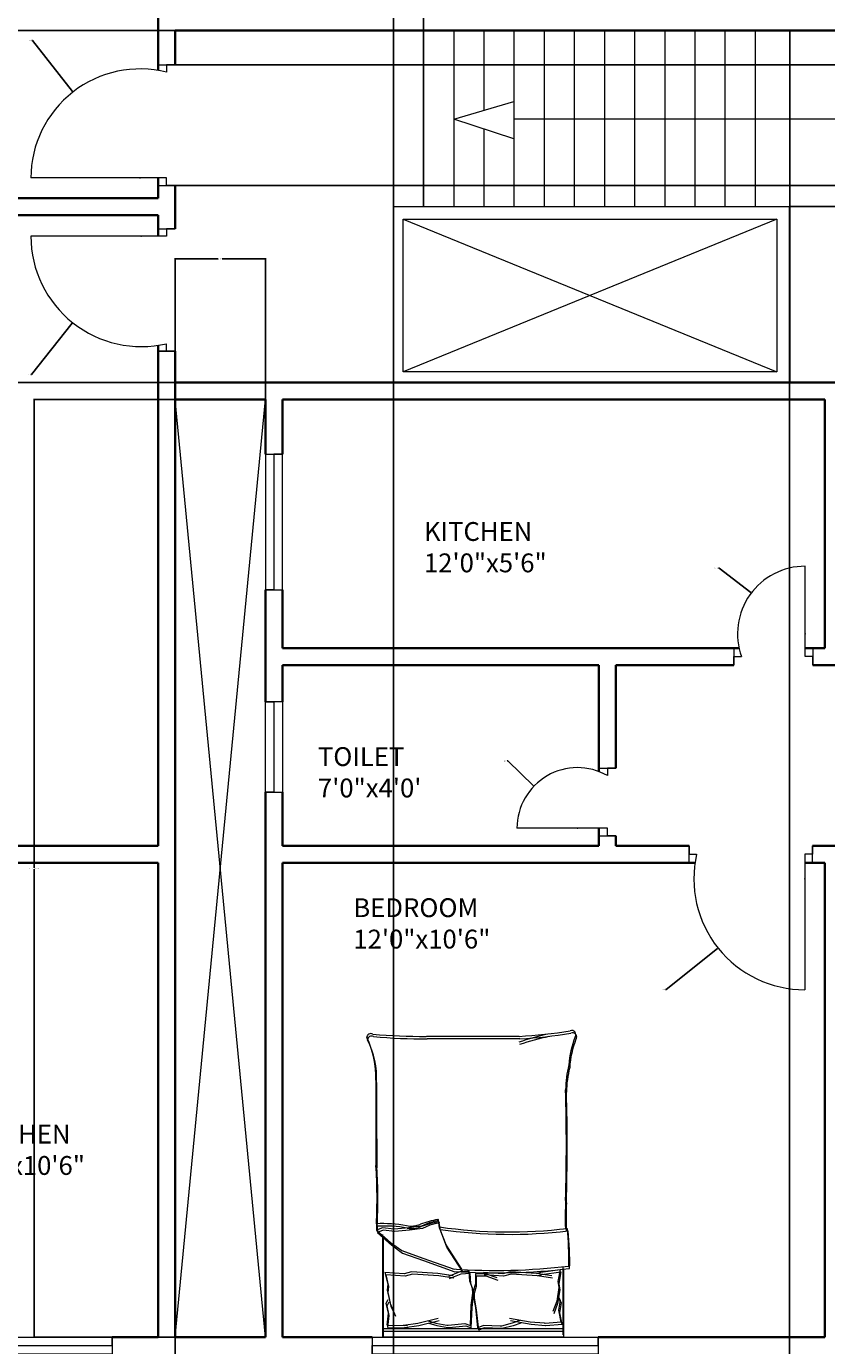
# Model space of a CAD drawing. Units: inches. Extents: x 1937 to 2996, y 1402 to 2323.
# Tile 3 of 10: x 2253 to 2466, y 1594 to 1944. Entities that reach past the tile are written whole.
import ezdxf

# ---------------------------------------------------------------- set-up
doc = ezdxf.new("R2010")
doc.units = ezdxf.units.IN
for name, color, linetype, lineweight in [('A-ANNO-DIMS', 2, 'Continuous', 18), ('A-AREA-IDEN', 7, 'Continuous', 18), ('A-DOOR', 11, 'Continuous', 18), ('A-FLOR-OPEN', 81, 'Continuous', 18), ('A-FLOR-STRS', 81, 'Continuous', 18), ('A-FURN', 8, 'Continuous', 13), ('A-GLAZ', 141, 'Continuous', 18), ('A-WALL', 7, 'Continuous', 35)]:
    doc.layers.add(name, color=color, linetype=linetype, lineweight=lineweight)
doc.styles.get("Standard").update_dxf_attribs({"font": 'arial.ttf'})
doc.dimstyles.get("Standard").update_dxf_attribs({"dimtxt": 0.18, "dimasz": 0.18, "dimexe": 0.18, "dimexo": 0.0625, "dimgap": 0.09, "dimtad": 0, "dimtih": 1, "dimtoh": 1, "dimdec": 4, "dimzin": 0, "dimdsep": 46, "dimtxsty": 'Standard', "dimcen": 0.09, "dimadec": 0, "dimazin": 0, "dimtfac": 1, "dimtdec": 4, "dimtofl": 0, "dimtmove": 0, "dimatfit": 3, "dimfxl": 1, "dimtolj": 1, "dimtzin": 0, "dimarcsym": 0})

# ---------------------------------------------------------------- blocks, each defined once
blk = doc.blocks.new('BED-DOUBLE')
for p, q in [((-24.01, -18.11), (-24.01, 0)), ((-24.01, -18.11), (-24.01, 0)), ((-24.01, 0), (24.01, 0)), ((23.78, 0), (23.78, -26.61)), ((23.78, 0), (23.78, -26.61)), ((24.01, 0), (24.01, -0.64)), ((-24.01, -1.53), (23.78, -1.53)), ((-24.01, -1.53), (23.78, -1.53)), ((-23.78, -18.75), (-23.78, -0.64)), ((-23.78, -18.75), (-23.78, -0.64)), ((-23.78, -2.17), (24.01, -2.17)), ((-23.78, -2.17), (24.01, -2.17)), ((-23.59, -3.34), (-19.3, -3.01)), ((-23.59, -3.34), (-19.31, -3.01)), ((-23.59, -3.32), (-23.01, -6.5)), ((-23.59, -3.32), (-23.01, -6.5)), ((-19.31, -3.01), (-19.2, -3.03)), ((-19.3, -3.01), (-19.2, -3.03)), ((-19.2, -3.03), (-15.38, -3.32)), ((-19.2, -3.03), (-15.38, -3.32)), ((-15.38, -3.32), (-9.88, -4.33)), ((-15.38, -3.32), (-9.88, -4.33)), ((-12.63, -3.75), (-10.61, -3.03)), ((-12.63, -3.75), (-10.61, -3.03)), ((-10.61, -3.03), (-7.71, -2.3)), ((-10.61, -3.03), (-7.71, -2.3)), ((-10.38, -3.67), (-7.49, -2.94)), ((-10.38, -3.67), (-7.49, -2.94)), ((-7.71, -2.3), (-7.39, -2.3)), ((-7.71, -2.3), (-7.39, -2.3)), ((-7.49, -2.94), (-7.16, -2.94)), ((-7.49, -2.94), (-7.16, -2.94)), ((-7.39, -2.3), (-2.95, -2.45)), ((-7.39, -2.3), (-2.95, -2.45)), ((-7.16, -2.94), (-2.72, -3.09)), ((-7.16, -2.94), (-2.72, -3.09)), ((-2.95, -2.45), (-1.5, -1.87)), ((-2.95, -2.45), (-1.5, -1.87)), ((-2.72, -3.09), (-1.27, -2.51)), ((-2.72, -3.09), (-1.27, -2.51)), ((-1.5, -1.87), (-0.92, -7.22)), ((-1.5, -1.87), (-0.92, -7.22)), ((-1.27, -2.51), (-0.7, -7.86)), ((-1.27, -2.51), (-0.7, -7.86)), ((0.49, -2.49), (0.25, -7.87)), ((0.49, -2.49), (0.25, -7.87)), ((0.72, -3.13), (0.48, -8.51)), ((0.72, -3.13), (0.48, -8.51)), ((1.97, -2.98), (0.49, -2.49)), ((1.97, -2.98), (0.49, -2.49)), ((2.2, -3.62), (0.72, -3.13)), ((2.2, -3.62), (0.72, -3.13)), ((6.4, -2.56), (1.97, -2.98)), ((6.4, -2.56), (1.97, -2.98)), ((6.63, -3.2), (2.2, -3.62)), ((6.63, -3.2), (2.2, -3.62)), ((6.72, -2.54), (6.4, -2.56)), ((6.72, -2.54), (6.4, -2.56)), ((6.95, -3.18), (6.63, -3.2)), ((6.95, -3.18), (6.63, -3.2)), ((9.65, -3.08), (6.72, -2.54)), ((9.65, -3.08), (6.72, -2.54)), ((9.88, -3.72), (6.95, -3.18)), ((9.88, -3.72), (6.95, -3.18)), ((14.43, -3.07), (9.01, -4.42)), ((14.43, -3.07), (9.01, -4.42)), ((11.72, -3.67), (9.65, -3.08)), ((11.72, -3.67), (9.65, -3.08)), ((18.23, -2.54), (14.43, -3.07)), ((18.23, -2.54), (14.43, -3.07)), ((18.46, -3.18), (14.66, -3.71)), ((18.46, -3.18), (14.66, -3.71)), ((22.63, -2.56), (17.23, -2.46)), ((17.23, -2.46), (18.23, -2.54)), ((22.63, -2.56), (17.23, -2.46)), ((17.23, -2.46), (18.23, -2.54)), ((22.86, -3.2), (17.45, -3.1)), ((17.45, -3.1), (18.46, -3.18)), ((22.86, -3.2), (17.45, -3.1)), ((17.45, -3.1), (18.46, -3.18)), ((22.63, -2.56), (22.25, -5.77)), ((22.63, -2.56), (22.25, -5.77)), ((22.86, -3.2), (22.48, -6.41)), ((22.86, -3.2), (22.48, -6.41)), ((24.01, -0.64), (24.01, -27.25)), ((24.01, -0.64), (24.01, -27.25)), ((-23.01, -6.5), (-23.45, -9.1)), ((-23.01, -6.5), (-23.45, -9.1)), ((-23.36, -3.98), (-19.08, -3.65)), ((-23.36, -3.98), (-19.08, -3.65)), ((-23.36, -3.96), (-22.78, -7.14)), ((-23.36, -3.96), (-22.78, -7.14)), ((-22.43, -8.96), (-21.42, -6.21)), ((-22.43, -8.96), (-21.42, -6.21)), ((-22.21, -9.59), (-21.19, -6.85)), ((-22.2, -9.59), (-21.19, -6.85)), ((-19.08, -3.65), (-18.97, -3.67)), ((-19.08, -3.65), (-18.97, -3.67)), ((-18.97, -3.67), (-15.15, -3.96)), ((-18.97, -3.67), (-15.15, -3.96)), ((-15.15, -3.96), (-9.65, -4.97)), ((-15.15, -3.96), (-9.65, -4.97)), ((-12.4, -4.39), (-10.38, -3.67)), ((-12.4, -4.39), (-10.38, -3.67)), ((14.66, -3.71), (9.24, -5.06)), ((14.66, -3.71), (9.24, -5.06)), ((11.94, -4.31), (9.88, -3.72)), ((11.94, -4.31), (9.88, -3.72)), ((21.83, -8.26), (20.64, -5.58)), ((21.82, -8.26), (20.64, -5.58)), ((22.05, -8.9), (20.87, -6.22)), ((22.05, -8.9), (20.87, -6.22)), ((22.25, -5.77), (22.84, -8.34)), ((22.25, -5.77), (22.84, -8.34)), ((22.48, -6.41), (23.07, -8.98)), ((22.48, -6.41), (23.07, -8.98)), ((-23.45, -9.1), (-22.87, -10.11)), ((-23.45, -9.1), (-22.87, -10.11)), ((-22.78, -7.14), (-23.22, -9.74)), ((-22.78, -7.14), (-23.22, -9.74)), ((-23.22, -9.74), (-22.64, -10.75)), ((-23.22, -9.74), (-22.64, -10.75)), ((-23.01, -12.57), (-22.43, -8.96)), ((-23.01, -12.57), (-22.43, -8.96)), ((-22.78, -13.21), (-22.2, -9.59)), ((-22.78, -13.21), (-22.21, -9.59)), ((-0.92, -7.22), (-0.35, -10.4)), ((-0.92, -7.22), (-0.35, -10.4)), ((-0.7, -7.86), (-0.12, -11.04)), ((-0.7, -7.86), (-0.12, -11.04)), ((-0.35, -10.4), (-0.35, -11.7)), ((-0.35, -10.4), (-0.35, -11.7)), ((0.25, -7.87), (-0.13, -11.08)), ((0.25, -7.87), (-0.13, -11.08)), ((0.48, -8.51), (0.1, -11.72)), ((0.48, -8.51), (0.1, -11.72)), ((22.63, -11.83), (21.82, -8.26)), ((22.63, -11.83), (21.83, -8.26)), ((22.86, -12.47), (22.05, -8.9)), ((22.86, -12.47), (22.05, -8.9)), ((22.84, -8.34), (22.33, -9.38)), ((22.84, -8.34), (22.33, -9.38)), ((23.07, -8.98), (22.56, -10.02)), ((23.07, -8.98), (22.56, -10.02)), ((-22.72, -14.16), (-23.01, -12.57)), ((-22.72, -14.16), (-23.01, -12.57)), ((-22.49, -14.8), (-22.78, -13.21)), ((-22.49, -14.8), (-22.78, -13.21)), ((-0.35, -11.7), (-0.92, -13.58)), ((-0.35, -11.7), (-0.92, -13.58)), ((-0.92, -13.58), (-0.92, -16.26)), ((-0.92, -13.58), (-0.92, -16.26)), ((-0.12, -12.34), (-0.7, -14.22)), ((-0.12, -12.34), (-0.7, -14.22)), ((-0.13, -11.08), (-0.05, -12.38)), ((-0.13, -11.08), (-0.05, -12.38)), ((-0.12, -11.04), (-0.12, -12.34)), ((-0.12, -11.04), (-0.12, -12.34)), ((-0.05, -12.38), (0.65, -14.22)), ((-0.05, -12.38), (0.65, -14.22)), ((0.1, -11.72), (0.18, -13.02)), ((0.1, -11.72), (0.18, -13.02)), ((0.18, -13.02), (0.87, -14.86)), ((0.18, -13.02), (0.87, -14.86)), ((22.44, -13.43), (22.63, -11.83)), ((22.44, -13.43), (22.63, -11.83)), ((23.21, -16.57), (22.44, -13.43)), ((23.21, -16.57), (22.44, -13.43)), ((22.67, -14.07), (22.86, -12.47)), ((22.67, -14.07), (22.86, -12.47)), ((-23.3, -17.34), (-22.72, -14.16)), ((-23.3, -17.34), (-22.72, -14.16)), ((-18.2, -16.62), (-23.3, -17.34)), ((-18.2, -16.62), (-23.3, -17.34)), ((-23.07, -17.98), (-22.49, -14.8)), ((-23.07, -17.98), (-22.49, -14.8)), ((-17.98, -17.26), (-23.07, -17.98)), ((-17.98, -17.26), (-23.07, -17.98)), ((-21.1, -15.63), (-17.07, -16.3)), ((-21.1, -15.63), (-17.07, -16.3)), ((-20.87, -16.27), (-16.84, -16.93)), ((-20.87, -16.27), (-16.84, -16.93)), ((-17.07, -16.3), (-18.2, -16.62)), ((-17.07, -16.3), (-18.2, -16.62)), ((-16.84, -16.93), (-17.98, -17.26)), ((-16.84, -16.93), (-17.98, -17.26)), ((-17.07, -16.3), (-10.06, -16.73)), ((-17.07, -16.3), (-10.06, -16.73)), ((-16.84, -16.93), (-9.83, -17.37)), ((-16.84, -16.93), (-9.83, -17.37)), ((-10.06, -16.73), (-8.1, -16.17)), ((-10.06, -16.73), (-8.1, -16.17)), ((-9.83, -17.37), (-7.87, -16.81)), ((-9.83, -17.37), (-7.87, -16.81)), ((-8.1, -16.17), (-2.97, -16.57)), ((-8.1, -16.17), (-2.97, -16.57)), ((-7.87, -16.81), (-2.74, -17.21)), ((-7.87, -16.81), (-2.74, -17.21)), ((-3.38, -16.26), (-6.53, -15.17)), ((-3.38, -16.26), (-6.53, -15.17)), ((-3.15, -16.9), (-6.3, -15.81)), ((-3.15, -16.9), (-6.3, -15.81)), ((-0.92, -16.26), (-3.38, -16.26)), ((-0.92, -16.26), (-3.38, -16.26)), ((-0.7, -16.9), (-3.15, -16.9)), ((-0.7, -16.9), (-3.15, -16.9)), ((-0.7, -14.22), (-0.7, -16.9)), ((-0.7, -14.22), (-0.7, -16.9)), ((0.65, -14.22), (0.81, -16.89)), ((0.65, -14.22), (0.81, -16.89)), ((0.81, -16.89), (3.27, -16.74)), ((0.81, -16.89), (3.27, -16.74)), ((0.87, -14.86), (1.04, -17.53)), ((0.87, -14.86), (1.04, -17.53)), ((1.04, -17.53), (3.49, -17.38)), ((1.04, -17.53), (3.49, -17.38)), ((2.77, -17.38), (6.97, -23.88)), ((2.77, -17.38), (6.96, -23.88)), ((3.27, -16.74), (6.34, -15.45)), ((3.27, -16.74), (6.34, -15.45)), ((3.49, -17.38), (6.56, -16.09)), ((3.49, -17.38), (6.56, -16.09)), ((13.16, -20.32), (4.82, -17.38)), ((13.16, -20.32), (4.82, -17.38)), ((5.08, -15.63), (9.11, -16.3)), ((5.08, -15.63), (9.11, -16.3)), ((5.31, -16.27), (9.34, -16.93)), ((5.31, -16.27), (9.34, -16.93)), ((9.11, -16.3), (16.12, -16.73)), ((9.11, -16.3), (16.12, -16.73)), ((9.34, -16.93), (16.35, -17.37)), ((9.34, -16.93), (16.35, -17.37)), ((16.12, -16.73), (18.08, -16.17)), ((16.12, -16.73), (18.08, -16.17)), ((16.35, -17.37), (18.31, -16.81)), ((16.35, -17.37), (18.31, -16.81)), ((18.08, -16.17), (23.21, -16.57)), ((18.08, -16.17), (23.21, -16.57)), ((18.31, -16.81), (23.44, -17.21)), ((18.31, -16.81), (23.44, -17.21)), ((23.44, -17.21), (22.67, -14.07)), ((23.44, -17.21), (22.67, -14.07)), ((3, -18.02), (7.19, -24.52)), ((3, -18.02), (7.19, -24.52)), ((13.39, -20.96), (5.05, -18.02)), ((13.39, -20.96), (5.05, -18.02)), ((18.74, -22.33), (13.16, -20.32)), ((18.74, -22.33), (13.16, -20.32)), ((18.96, -22.97), (13.39, -20.96)), ((18.96, -22.97), (13.39, -20.96)), ((6.96, -23.88), (8.67, -28.37)), ((6.97, -23.88), (8.67, -28.37)), ((7.19, -24.52), (8.9, -29)), ((7.19, -24.52), (8.9, -29)), ((21.68, -24.5), (18.74, -22.33)), ((21.68, -24.5), (18.74, -22.33)), ((21.91, -25.13), (18.96, -22.97)), ((21.91, -25.13), (18.96, -22.97)), ((25.38, -27.75), (21.68, -24.5)), ((25.38, -27.75), (21.68, -24.5)), ((25.61, -28.39), (21.91, -25.13)), ((25.61, -28.39), (21.91, -25.13)), ((23.85, -28.37), (25.38, -27.75)), ((23.85, -28.37), (25.38, -27.75)), ((25.46, -29.49), (25.38, -27.75, 3.87)), ((25.46, -29.49), (25.38, -27.75, 3.87)), ((8.67, -28.37), (8.98, -30.38)), ((8.67, -28.37), (8.98, -30.38)), ((8.9, -29), (9.21, -31.02)), ((8.9, -29), (9.21, -31.02)), ((8.98, -30.38), (11.46, -29.76)), ((8.98, -30.38), (11.46, -29.76)), ((9.21, -31.02), (11.68, -30.4)), ((9.21, -31.02), (11.68, -30.4)), ((11.46, -29.76), (13.47, -28.83)), ((11.46, -29.76), (13.47, -28.83)), ((11.68, -30.4), (13.7, -29.47)), ((11.68, -30.4), (13.7, -29.47)), ((13.47, -28.83), (16.88, -28.37)), ((13.47, -28.83), (16.88, -28.37)), ((13.7, -29.47), (17.11, -29)), ((13.7, -29.47), (17.1, -29)), ((16.88, -28.37), (20.75, -28.06)), ((16.88, -28.37), (20.75, -28.06)), ((17.1, -29), (20.98, -28.69)), ((17.11, -29), (20.98, -28.69)), ((20.75, -28.06), (23.85, -28.37)), ((20.75, -28.06), (23.85, -28.37)), ((20.98, -28.69), (24.07, -29)), ((20.98, -28.69), (24.07, -29)), ((24.07, -29), (25.61, -28.39)), ((24.07, -29), (25.61, -28.39)), ((25.69, -30.13), (25.61, -28.39, 3.87)), ((25.69, -30.13), (25.61, -28.39, 3.87)), ((-12.42, -79.25), (12.19, -79.25)), ((-12.42, -79.25), (12.19, -79.25)), ((-12.19, -79.88), (12.42, -79.88)), ((-12.19, -79.88), (12.42, -79.88))]:
    blk.add_line(p, q)
for centre, radius, start, end in [((-6.13, -182.05), 164.97, 86.0865, 96.7821), ((-6.13, -182.05), 164.97, 86.0865, 96.7821), ((57.68, -20.1), 83.31, 178.7218, 185.604), ((57.68, -20.1), 83.31, 178.7218, 185.604), ((57.91, -20.74), 83.31, 178.7218, 185.604), ((57.91, -20.74), 83.31, 178.7218, 185.604), ((-5.9, -182.69), 164.97, 86.0865, 96.7821), ((-5.9, -182.69), 164.97, 86.0865, 96.7821), ((-9.73, -156.32), 129.02, 81.7845, 96.9006), ((-9.73, -156.32), 129.02, 81.7845, 96.9006), ((-9.5, -156.96), 129.02, 81.7845, 96.9006), ((-9.5, -156.96), 129.02, 81.7845, 96.9006), ((-194.79, -31.17), 170.11, 358.4762, 1.0082), ((-194.79, -31.17), 170.11, 358.4762, 1.0082), ((-194.56, -31.81), 170.11, 358.4762, 1.0082), ((-194.56, -31.81), 170.11, 358.4762, 1.0082), ((9.15, -30.44), 0.185, 160.2464, 271.1377), ((9.15, -30.44), 0.185, 160.2464, 271.1377), ((3.67, -1.48), 29.65, 280.6617, 289.8806), ((3.67, -1.48), 29.65, 280.6617, 289.8806), ((9.38, -31.08), 0.185, 160.2464, 271.1377), ((9.38, -31.08), 0.185, 160.2464, 271.1377), ((3.9, -2.12), 29.65, 280.6617, 289.8806), ((3.9, -2.12), 29.65, 280.6617, 289.8806), ((16.26, -35.07), 6.22, 78.6608, 113.7384), ((16.26, -35.07), 6.22, 78.6608, 113.7384), ((16.49, -35.71), 6.22, 78.6608, 113.7384), ((16.49, -35.71), 6.22, 78.6608, 113.7384), ((23.84, 6.66), 36.18, 259.8763, 272.5657), ((23.84, 6.66), 36.18, 259.8763, 272.5657), ((24.07, 6.02), 36.18, 259.8763, 272.5657), ((24.07, 6.02), 36.18, 259.8763, 272.5657), ((154.78, -36.32), 129.5, 176.9791, 183.8365), ((154.78, -36.32), 129.5, 176.9791, 183.8365), ((155.01, -36.95), 129.5, 176.9791, 183.8365), ((155.01, -36.95), 129.5, 176.9791, 183.8365), ((457.34, -50.61), 482.31, 178.2277, 181.7185), ((457.34, -50.61), 482.31, 178.2277, 181.7185), ((457.57, -51.25), 482.31, 178.2277, 181.7185), ((457.57, -51.25), 482.31, 178.2277, 181.7185), ((-4536.23, -67.82), 4561.86, 0.00217, 0.28689), ((-4536.23, -67.82), 4561.86, 0.00217, 0.28689), ((-4536, -68.46), 4561.86, 0.00217, 0.28689), ((-4536, -68.46), 4561.86, 0.00217, 0.28689), ((-54.38, -64.52), 29.63, 346.0648, 358.9113), ((-54.38, -64.52), 29.63, 346.0648, 358.9113), ((-54.16, -65.15), 29.63, 346.0648, 358.9113), ((-54.16, -65.15), 29.63, 346.0648, 358.9113), ((48.67, -68.67), 23.07, 177.4714, 206.4681), ((48.67, -68.67), 23.07, 177.4714, 206.4681), ((48.9, -69.31), 23.07, 177.4714, 206.4681), ((48.9, -69.31), 23.07, 177.4714, 206.4681), ((-49.14, -70.28), 23.56, 337.9751, 356.652), ((-49.14, -70.28), 23.56, 337.9751, 356.652), ((-48.92, -70.91), 23.56, 337.9751, 356.652), ((-48.92, -70.91), 23.56, 337.9751, 356.652), ((-26.4, -79.72), 1.09, 146.1736, 293.4781), ((-26.4, -79.72), 1.09, 146.1736, 293.4781), ((-26.17, -80.36), 1.09, 146.1736, 293.4781), ((-26.17, -80.36), 1.09, 146.1736, 293.4781), ((-6.06, -200.84), 121.76, 92.9958, 99.4091), ((-6.06, -200.84), 121.76, 92.9958, 99.4091), ((-5.83, -201.48), 121.76, 92.9958, 99.4091), ((-5.83, -201.48), 121.76, 92.9958, 99.4091), ((-44.71, 23.71), 106.46, 283.3832, 287.7053), ((-44.71, 23.71), 106.46, 283.3832, 287.7053), ((-44.48, 23.07), 106.46, 283.3832, 287.7053), ((-44.48, 23.07), 106.46, 283.3832, 287.7053), ((13.67, -212.28), 133.04, 84.4998, 90.6351), ((13.67, -212.28), 133.04, 84.4998, 90.6351), ((13.9, -212.92), 133.04, 84.4998, 90.6351), ((13.9, -212.92), 133.04, 84.4998, 90.6351), ((26.93, -78.87), 1.1, 242.6588, 356.02), ((26.93, -78.87), 1.1, 242.6588, 356.02), ((27.15, -79.51), 1.1, 242.6588, 356.02), ((27.15, -79.51), 1.1, 242.6588, 356.02)]:
    blk.add_arc(centre, radius, start, end)
blk = doc.blocks.new('WINDOW-60IN')
for p, q in [((0, 2.25), (0, -2.25)), ((0, 2.25), (60, 2.25)), ((0, -2.25), (0, 0)), ((0, 0), (60, 0)), ((60, 0), (60, 2.25)), ((60, 2.25), (60, -2.25)), ((60, -2.25), (0, -2.25))]:
    blk.add_line(p, q)
blk = doc.blocks.new('WINDOW-36IN')
for p, q in [((0, 2.25), (0, -2.25)), ((0, 2.25), (36, 2.25)), ((36, 0), (36, 2.25)), ((36, 2.25), (36, -2.25)), ((0, -2.25), (0, 0)), ((0, 0), (36, 0)), ((36, -2.25), (0, -2.25))]:
    blk.add_line(p, q)
blk = doc.blocks.new('WINDOW-24IN-JAMB-B')
for p, q in [((0, -2.25), (0, 2.25)), ((0, 2.25), (0, 0)), ((24, 2.25), (0, 2.25)), ((0, 0), (24, 0)), ((24, 0), (24, 2.25)), ((24, 2.25), (24, -2.25)), ((0, -2.25), (24, -2.25))]:
    blk.add_line(p, q)
blk = doc.blocks.new('VOID-MARK-24X249')
for p, q in [((24, 249), (0, 0)), ((0, 249), (24, 0))]:
    blk.add_line(p, q)
blk = doc.blocks.new('*D21')
at = {"layer": 'A-ANNO-DIMS', "color": 0, "lineweight": -2, "transparency": 16777216}
for p, q in [((2292.58, 1844.81), (2255.12, 1844.81)), ((2255.3, 1844.63), (2255.3, 1720.49)), ((2255.3, 1595.99), (2255.3, 1720.12)), ((2292.58, 1595.81), (2255.12, 1595.81))]:
    blk.add_line(p, q, dxfattribs=at)
at = {"layer": 'A-ANNO-DIMS', "color": 0, "transparency": 16777216}
for points in [[(2255.27, 1844.63), (2255.33, 1844.63), (2255.3, 1844.81)], [(2255.27, 1595.99), (2255.33, 1595.99), (2255.3, 1595.81)]]:
    blk.add_solid(points, dxfattribs=at)
at = {"layer": 'Defpoints', "color": 0, "transparency": 16777216}
for p in [(2292.65, 1844.81), (2255.3, 1595.81), (2292.65, 1595.81)]:
    blk.add_point(p, dxfattribs=at)
at = {"layer": 'A-ANNO-DIMS', "color": 0, "transparency": 16777216, "insert": (2255.3, 1720.31), "char_height": 0.18, "attachment_point": 5}
blk.add_mtext('\\A1;FLOOR VOID 249 TYP.', dxfattribs=at)
blk = doc.blocks.new('*D22')
at = {"layer": 'A-ANNO-DIMS', "color": 0, "lineweight": -2, "transparency": 16777216}
for p, q in [((2292.65, 1844.87), (2292.65, 1882.34)), ((2292.83, 1882.16), (2304.12, 1882.16)), ((2316.47, 1882.16), (2305.18, 1882.16)), ((2316.65, 1844.87), (2316.65, 1882.34))]:
    blk.add_line(p, q, dxfattribs=at)
at = {"layer": 'A-ANNO-DIMS', "color": 0, "transparency": 16777216}
for points in [[(2292.83, 1882.19), (2292.83, 1882.13), (2292.65, 1882.16)], [(2316.47, 1882.19), (2316.47, 1882.13), (2316.65, 1882.16)]]:
    blk.add_solid(points, dxfattribs=at)
at = {"layer": 'Defpoints', "color": 0, "transparency": 16777216}
for p in [(2292.65, 1882.16), (2292.65, 1844.81), (2316.65, 1844.81)]:
    blk.add_point(p, dxfattribs=at)
at = {"layer": 'A-ANNO-DIMS', "color": 0, "transparency": 16777216, "insert": (2304.65, 1882.16), "char_height": 0.18, "attachment_point": 5}
blk.add_mtext('\\A1;24 TYP.', dxfattribs=at)
blk = doc.blocks.new('*D23')
at = {"layer": 'A-ANNO-DIMS', "color": 0, "lineweight": -2, "transparency": 16777216}
for p, q in [((2010.65, 1769.24), (2010.65, 1508.98)), ((2924.15, 1769.24), (2924.15, 1508.98)), ((2010.83, 1509.16), (2467, 1509.16)), ((2923.97, 1509.16), (2467.79, 1509.16))]:
    blk.add_line(p, q, dxfattribs=at)
at = {"layer": 'A-ANNO-DIMS', "color": 0, "transparency": 16777216}
for points in [[(2010.83, 1509.19), (2010.83, 1509.13), (2010.65, 1509.16)], [(2923.97, 1509.19), (2923.97, 1509.13), (2924.15, 1509.16)]]:
    blk.add_solid(points, dxfattribs=at)
at = {"layer": 'Defpoints', "color": 0, "transparency": 16777216}
for p in [(2010.65, 1769.31), (2924.15, 1769.31), (2924.15, 1509.16)]:
    blk.add_point(p, dxfattribs=at)
at = {"layer": 'A-ANNO-DIMS', "color": 0, "transparency": 16777216, "insert": (2467.4, 1509.16), "char_height": 0.18, "attachment_point": 5}
blk.add_mtext('\\A1;913.5', dxfattribs=at)
blk = doc.blocks.new('*D32')
at = {"layer": 'A-ANNO-DIMS', "color": 0, "lineweight": -2, "transparency": 16777216}
for p, q in [((2350.55, 1942.81), (1964.32, 1942.81)), ((1964.5, 1942.63), (1964.5, 1896.24)), ((1964.5, 1849.49), (1964.5, 1895.87)), ((2350.55, 1849.31), (1964.32, 1849.31))]:
    blk.add_line(p, q, dxfattribs=at)
at = {"layer": 'A-ANNO-DIMS', "color": 0, "transparency": 16777216}
for points in [[(1964.47, 1942.63), (1964.53, 1942.63), (1964.5, 1942.81)], [(1964.47, 1849.49), (1964.53, 1849.49), (1964.5, 1849.31)]]:
    blk.add_solid(points, dxfattribs=at)
at = {"layer": 'Defpoints', "color": 0, "transparency": 16777216}
for p in [(1964.5, 1942.81), (2350.61, 1942.81), (2350.61, 1849.31)]:
    blk.add_point(p, dxfattribs=at)
at = {"layer": 'A-ANNO-DIMS', "color": 0, "transparency": 16777216, "insert": (1964.5, 1896.06), "char_height": 0.18, "attachment_point": 5}
blk.add_mtext('\\A1;93.5', dxfattribs=at)
blk = doc.blocks.new('*D33')
at = {"layer": 'A-ANNO-DIMS', "color": 0, "lineweight": -2, "transparency": 16777216}
for p, q in [((2292.65, 1849.24), (2292.65, 1508.98)), ((2350.61, 1849.24), (2350.61, 1508.98)), ((2292.83, 1509.16), (2321.24, 1509.16)), ((2350.43, 1509.16), (2322.02, 1509.16))]:
    blk.add_line(p, q, dxfattribs=at)
at = {"layer": 'A-ANNO-DIMS', "color": 0, "transparency": 16777216}
for points in [[(2292.83, 1509.19), (2292.83, 1509.13), (2292.65, 1509.16)], [(2350.43, 1509.19), (2350.43, 1509.13), (2350.61, 1509.16)]]:
    blk.add_solid(points, dxfattribs=at)
at = {"layer": 'Defpoints', "color": 0, "transparency": 16777216}
for p in [(2292.65, 1849.31), (2350.61, 1849.31), (2350.61, 1509.16)]:
    blk.add_point(p, dxfattribs=at)
at = {"layer": 'A-ANNO-DIMS', "color": 0, "transparency": 16777216, "insert": (2321.63, 1509.16), "char_height": 0.18, "attachment_point": 5}
blk.add_mtext('\\A1;57.96', dxfattribs=at)
blk = doc.blocks.new('*D34')
at = {"layer": 'A-ANNO-DIMS', "color": 0, "lineweight": -2, "transparency": 16777216}
for p, q in [((2350.61, 1849.24), (2350.61, 1508.98)), ((2561.65, 1849.24), (2561.65, 1508.98)), ((2350.79, 1509.16), (2455.66, 1509.16)), ((2561.47, 1509.16), (2456.59, 1509.16))]:
    blk.add_line(p, q, dxfattribs=at)
at = {"layer": 'A-ANNO-DIMS', "color": 0, "transparency": 16777216}
for points in [[(2350.79, 1509.19), (2350.79, 1509.13), (2350.61, 1509.16)], [(2561.47, 1509.19), (2561.47, 1509.13), (2561.65, 1509.16)]]:
    blk.add_solid(points, dxfattribs=at)
at = {"layer": 'Defpoints', "color": 0, "transparency": 16777216}
for p in [(2350.61, 1849.31), (2561.65, 1849.31), (2561.65, 1509.16)]:
    blk.add_point(p, dxfattribs=at)
at = {"layer": 'A-ANNO-DIMS', "color": 0, "transparency": 16777216, "insert": (2456.13, 1509.16), "char_height": 0.18, "attachment_point": 5}
blk.add_mtext('\\A1;211.04', dxfattribs=at)
blk = doc.blocks.new('*D36')
at = {"layer": 'A-ANNO-DIMS', "color": 0, "lineweight": -2, "transparency": 16777216}
for p, q in [((2350.61, 1896.12), (2350.61, 2283.14)), ((2350.79, 2282.96), (2354.46, 2282.96)), ((2358.43, 2282.96), (2354.76, 2282.96)), ((2358.61, 1896.12), (2358.61, 2283.14))]:
    blk.add_line(p, q, dxfattribs=at)
at = {"layer": 'A-ANNO-DIMS', "color": 0, "transparency": 16777216}
for points in [[(2350.79, 2282.99), (2350.79, 2282.93), (2350.61, 2282.96)], [(2358.43, 2282.99), (2358.43, 2282.93), (2358.61, 2282.96)]]:
    blk.add_solid(points, dxfattribs=at)
at = {"layer": 'Defpoints', "color": 0, "transparency": 16777216}
for p in [(2358.61, 2282.96), (2350.61, 1896.06), (2358.61, 1896.06)]:
    blk.add_point(p, dxfattribs=at)
at = {"layer": 'A-ANNO-DIMS', "color": 0, "transparency": 16777216, "insert": (2354.61, 2282.96), "char_height": 0.18, "attachment_point": 5}
blk.add_mtext('\\A1;8', dxfattribs=at)
blk = doc.blocks.new('*D37')
at = {"layer": 'A-ANNO-DIMS', "color": 0, "lineweight": -2, "transparency": 16777216}
for p, q in [((2455.84, 1896.06), (2970.48, 1896.06)), ((2970.3, 1895.88), (2970.3, 1872.86)), ((2970.3, 1849.49), (2970.3, 1872.5)), ((2455.84, 1849.31), (2970.48, 1849.31))]:
    blk.add_line(p, q, dxfattribs=at)
at = {"layer": 'A-ANNO-DIMS', "color": 0, "transparency": 16777216}
for points in [[(2970.27, 1895.88), (2970.33, 1895.88), (2970.3, 1896.06)], [(2970.27, 1849.49), (2970.33, 1849.49), (2970.3, 1849.31)]]:
    blk.add_solid(points, dxfattribs=at)
at = {"layer": 'Defpoints', "color": 0, "transparency": 16777216}
for p in [(2455.77, 1896.06), (2455.77, 1849.31), (2970.3, 1849.31)]:
    blk.add_point(p, dxfattribs=at)
at = {"layer": 'A-ANNO-DIMS', "color": 0, "transparency": 16777216, "insert": (2970.3, 1872.68), "char_height": 0.18, "attachment_point": 5}
blk.add_mtext('\\A1;46.75', dxfattribs=at)
blk = doc.blocks.new('*D38')
at = {"layer": 'A-ANNO-DIMS', "color": 0, "lineweight": -2, "transparency": 16777216}
for p, q in [((2350.61, 1895.99), (2350.61, 1508.98)), ((2455.77, 1895.99), (2455.77, 1508.98)), ((2350.79, 1509.16), (2402.74, 1509.16)), ((2455.59, 1509.16), (2403.65, 1509.16))]:
    blk.add_line(p, q, dxfattribs=at)
at = {"layer": 'A-ANNO-DIMS', "color": 0, "transparency": 16777216}
for points in [[(2350.79, 1509.19), (2350.79, 1509.13), (2350.61, 1509.16)], [(2455.59, 1509.19), (2455.59, 1509.13), (2455.77, 1509.16)]]:
    blk.add_solid(points, dxfattribs=at)
at = {"layer": 'Defpoints', "color": 0, "transparency": 16777216}
for p in [(2350.61, 1896.06), (2455.77, 1896.06), (2455.77, 1509.16)]:
    blk.add_point(p, dxfattribs=at)
at = {"layer": 'A-ANNO-DIMS', "color": 0, "transparency": 16777216, "insert": (2403.19, 1509.16), "char_height": 0.18, "attachment_point": 5}
blk.add_mtext('\\A1;105.16', dxfattribs=at)
blk = doc.blocks.new('*D50')
at = {"layer": 'A-ANNO-DIMS', "color": 0, "lineweight": -2, "transparency": 16777216}
for p, q in [((2292.71, 1933.76), (2970.48, 1933.76)), ((2970.3, 1933.58), (2970.3, 1917.9)), ((2970.3, 1901.85), (2970.3, 1917.53)), ((2292.71, 1901.67), (2970.48, 1901.67))]:
    blk.add_line(p, q, dxfattribs=at)
at = {"layer": 'A-ANNO-DIMS', "color": 0, "transparency": 16777216}
for points in [[(2970.27, 1933.58), (2970.33, 1933.58), (2970.3, 1933.76)], [(2970.27, 1901.85), (2970.33, 1901.85), (2970.3, 1901.67)]]:
    blk.add_solid(points, dxfattribs=at)
at = {"layer": 'Defpoints', "color": 0, "transparency": 16777216}
for p in [(2292.65, 1933.76), (2970.3, 1933.76), (2292.65, 1901.67)]:
    blk.add_point(p, dxfattribs=at)
at = {"layer": 'A-ANNO-DIMS', "color": 0, "transparency": 16777216, "insert": (2970.3, 1917.71), "char_height": 0.18, "attachment_point": 5}
blk.add_mtext('\\A1;32.085', dxfattribs=at)
blk = doc.blocks.new('*D58')
at = {"layer": 'A-ANNO-DIMS', "color": 0, "lineweight": -2, "transparency": 16777216}
for p, q in [((2459.73, 1717.53), (2459.91, 1717.53)), ((2459.82, 1717.44), (2459.82, 1717.62)), ((2422.96, 1688.11), (2436.64, 1699.03)), ((2422.78, 1688.11), (2422.96, 1688.11))]:
    blk.add_line(p, q, dxfattribs=at)
at = {"layer": 'A-ANNO-DIMS', "color": 0, "transparency": 16777216}
blk.add_solid([(2436.63, 1699.05), (2436.66, 1699), (2436.78, 1699.14)], dxfattribs=at)
at = {"layer": 'Defpoints', "color": 0, "transparency": 16777216}
for p in [(2459.82, 1717.53), (2436.78, 1699.14)]:
    blk.add_point(p, dxfattribs=at)
at = {"layer": 'A-ANNO-DIMS', "color": 0, "transparency": 16777216, "insert": (2422.23, 1688.11), "char_height": 0.18, "attachment_point": 5}
blk.add_mtext('\\A1;R29.473', dxfattribs=at)
blk = doc.blocks.new('*D60')
at = {"layer": 'A-ANNO-DIMS', "color": 0, "lineweight": -2, "transparency": 16777216}
for p, q in [((2283.6, 1888.18), (2283.78, 1888.18)), ((2283.69, 1888.09), (2283.69, 1888.27)), ((2254.59, 1851.44), (2265.39, 1865.07)), ((2254.41, 1851.44), (2254.59, 1851.44))]:
    blk.add_line(p, q, dxfattribs=at)
at = {"layer": 'A-ANNO-DIMS', "color": 0, "transparency": 16777216}
blk.add_solid([(2265.37, 1865.09), (2265.41, 1865.05), (2265.5, 1865.21)], dxfattribs=at)
at = {"layer": 'Defpoints', "color": 0, "transparency": 16777216}
for p in [(2283.69, 1888.18), (2265.5, 1865.21)]:
    blk.add_point(p, dxfattribs=at)
at = {"layer": 'A-ANNO-DIMS', "color": 0, "transparency": 16777216, "insert": (2253.86, 1851.44), "char_height": 0.18, "attachment_point": 5}
blk.add_mtext('\\A1;R29.293', dxfattribs=at)
blk = doc.blocks.new('*D62')
at = {"layer": 'A-ANNO-DIMS', "color": 0, "lineweight": -2, "transparency": 16777216}
for p, q in [((2254.68, 1940.2), (2254.86, 1940.2)), ((2254.86, 1940.2), (2265.43, 1926.64)), ((2283.26, 1903.67), (2283.44, 1903.67)), ((2283.35, 1903.58), (2283.35, 1903.76))]:
    blk.add_line(p, q, dxfattribs=at)
at = {"layer": 'A-ANNO-DIMS', "color": 0, "transparency": 16777216}
blk.add_solid([(2265.46, 1926.66), (2265.41, 1926.62), (2265.54, 1926.5)], dxfattribs=at)
at = {"layer": 'Defpoints', "color": 0, "transparency": 16777216}
for p in [(2265.54, 1926.5), (2283.35, 1903.67)]:
    blk.add_point(p, dxfattribs=at)
at = {"layer": 'A-ANNO-DIMS', "color": 0, "transparency": 16777216, "insert": (2254.13, 1940.2), "char_height": 0.18, "attachment_point": 5}
blk.add_mtext('\\A1;R28.955', dxfattribs=at)
blk = doc.blocks.new('*D84')
at = {"layer": 'A-ANNO-DIMS', "color": 0, "lineweight": -2, "transparency": 16777216}
for p, q in [((2380.77, 1748.83), (2380.95, 1748.83)), ((2380.95, 1748.83), (2387.76, 1742.26)), ((2399.37, 1730.99), (2399.55, 1730.99)), ((2399.46, 1730.9), (2399.46, 1731.08))]:
    blk.add_line(p, q, dxfattribs=at)
at = {"layer": 'A-ANNO-DIMS', "color": 0, "transparency": 16777216}
blk.add_solid([(2387.79, 1742.29), (2387.74, 1742.24), (2387.89, 1742.14)], dxfattribs=at)
at = {"layer": 'Defpoints', "color": 0, "transparency": 16777216}
for p in [(2387.89, 1742.14), (2399.46, 1730.99)]:
    blk.add_point(p, dxfattribs=at)
at = {"layer": 'A-ANNO-DIMS', "color": 0, "transparency": 16777216, "insert": (2380.22, 1748.83), "char_height": 0.18, "attachment_point": 5}
blk.add_mtext('\\A1;R16.067', dxfattribs=at)
blk = doc.blocks.new('*D85')
at = {"layer": 'A-ANNO-DIMS', "color": 0, "lineweight": -2, "transparency": 16777216}
for p, q in [((2436.89, 1800.08), (2437.07, 1800.08)), ((2437.07, 1800.08), (2445.49, 1793.62)), ((2459.82, 1782.56), (2460, 1782.56)), ((2459.91, 1782.47), (2459.91, 1782.65))]:
    blk.add_line(p, q, dxfattribs=at)
at = {"layer": 'A-ANNO-DIMS', "color": 0, "transparency": 16777216}
blk.add_solid([(2445.51, 1793.65), (2445.48, 1793.6), (2445.64, 1793.51)], dxfattribs=at)
at = {"layer": 'Defpoints', "color": 0, "transparency": 16777216}
for p in [(2445.64, 1793.51), (2459.91, 1782.56)]:
    blk.add_point(p, dxfattribs=at)
at = {"layer": 'A-ANNO-DIMS', "color": 0, "transparency": 16777216, "insert": (2436.34, 1800.08), "char_height": 0.18, "attachment_point": 5}
blk.add_mtext('\\A1;R17.992', dxfattribs=at)

msp = doc.modelspace()

# ---------------------------------------------------------------- linework, layer by layer
at = {"layer": 'A-DOOR'}
for p, q in [((2288.1473, 1933.7562), (2292.6473, 1933.7562)), ((2292.6473, 1933.7562), (2290.3973, 1933.7562)), ((2290.3973, 1933.7562), (2290.3973, 1931.7562)), ((2290.3973, 1903.671), (2254.3973, 1903.671)), ((2290.3973, 1901.671), (2290.3973, 1903.671)), ((2288.1473, 1901.671), (2292.6473, 1901.671)), ((2292.6473, 1901.671), (2290.3973, 1901.671)), ((2288.1473, 1890.1765), (2292.6473, 1890.1765)), ((2292.6473, 1890.1765), (2290.3973, 1890.1765)), ((2290.3973, 1890.1765), (2290.3973, 1888.1765)), ((2290.3973, 1888.1765), (2254.3973, 1888.1765)), ((2292.6473, 1857.6611), (2288.1473, 1857.6611)), ((2288.1473, 1857.6611), (2292.6473, 1857.6611)), ((2290.3973, 1857.6611), (2290.3973, 1859.6611)), ((2459.9145, 1776.5561), (2459.9145, 1800.5561)), ((2440.9551, 1778.8061), (2440.9551, 1774.3061)), ((2440.9551, 1774.3061), (2440.9551, 1776.5561)), ((2440.9551, 1776.5561), (2442.9551, 1776.5561)), ((2461.9146, 1776.5561), (2459.9145, 1776.5561)), ((2461.9146, 1778.8061), (2461.9146, 1774.3061)), ((2461.9146, 1774.3061), (2461.9146, 1776.5561)), ((2405.1473, 1746.9636), (2409.6473, 1746.9636)), ((2409.6473, 1746.9636), (2407.3973, 1746.9636)), ((2407.3973, 1746.9636), (2407.3973, 1744.9636)), ((2407.3973, 1730.9908), (2383.3973, 1730.9908)), ((2407.3973, 1728.9908), (2407.3973, 1730.9908)), ((2405.1473, 1728.9908), (2409.6473, 1728.9908)), ((2409.6473, 1728.9908), (2407.3973, 1728.9908)), ((2429.0756, 1721.8061), (2429.0756, 1726.3061)), ((2429.0756, 1726.3061), (2429.0756, 1724.0561)), ((2429.0756, 1724.0561), (2431.0756, 1724.0561)), ((2461.8174, 1724.0561), (2459.8174, 1724.0561)), ((2459.8174, 1724.0561), (2459.8174, 1688.0561)), ((2461.8174, 1721.8061), (2461.8174, 1726.3061)), ((2461.8174, 1726.3061), (2461.8174, 1724.0561))]:
    msp.add_line(p, q, dxfattribs=at)
for centre, radius, start, end in [((2283.3525, 1903.671), 28.9552, 75.918665, 180), ((2283.6908, 1888.1765), 29.2935, 180, 283.234808), ((2459.9145, 1782.564), 17.9921, 90, 199.506737), ((2399.4648, 1730.9908), 16.0675, 60.41593, 180), ((2459.8174, 1717.5296), 29.4735, 167.20659, 270)]:
    msp.add_arc(centre, radius, start, end, dxfattribs=at)
at = {"layer": 'A-FLOR-OPEN'}
for p, q in [((2452.3737, 1892.7665), (2353.1608, 1852.1918)), ((2353.1608, 1892.7665), (2452.3737, 1852.1918))]:
    msp.add_line(p, q, dxfattribs=at)
msp.add_lwpolyline([(2353.1608, 1892.7665), (2452.3737, 1892.7665), (2452.3737, 1852.1918), (2353.1608, 1852.1918)], close=True, dxfattribs=at)
at = {"layer": 'A-FLOR-STRS'}
for p, q in [((2350.6104, 1942.8061), (2350.6104, 1849.3061)), ((2350.6104, 1942.8061), (2358.6104, 1942.8061)), ((2358.6104, 1942.8061), (2358.6104, 1896.0561)), ((2366.6104, 1942.8061), (2366.6104, 1896.0561)), ((2374.6104, 1942.8061), (2374.6104, 1921.6177)), ((2382.6104, 1942.8061), (2382.6104, 1896.0561)), ((2390.6104, 1942.8061), (2390.6104, 1896.0561)), ((2398.6104, 1942.8061), (2398.6104, 1896.0561)), ((2406.6104, 1942.8061), (2406.6104, 1896.0561)), ((2414.6104, 1942.8061), (2414.6104, 1896.0561)), ((2422.6104, 1942.8061), (2422.6104, 1896.0561)), ((2430.6104, 1942.8061), (2430.6104, 1896.0561)), ((2438.6104, 1942.8061), (2438.6104, 1896.0561)), ((2446.6104, 1942.8061), (2446.6104, 1896.0561)), ((2455.7744, 1896.0561), (2455.7744, 1942.8061)), ((2455.7744, 1942.8061), (2455.7744, 1849.3061)), ((2366.6104, 1919.2771), (2382.6104, 1923.9583)), ((2382.6104, 1923.9583), (2382.6104, 1914.0234)), ((2382.6104, 1914.0234), (2366.6104, 1919.2771)), ((2374.6104, 1916.6502), (2374.6104, 1896.0561)), ((2572.1291, 1919.2771), (2382.6104, 1919.2771)), ((2350.6104, 1849.3061), (2350.6104, 1896.0561)), ((2350.6104, 1896.0561), (2455.7744, 1896.0561))]:
    msp.add_line(p, q, dxfattribs=at)
for p in [(2358.6104, 1921.7544), (2358.6104, 1915.5474), (2358.6104, 1913.6583)]:
    msp.add_point(p, dxfattribs=at)
at = {"layer": 'A-WALL'}
for p, q in [((2288.1473, 2065.8061), (2288.1473, 1932.2265)), ((2292.6473, 1942.8061), (2316.6473, 1942.8061)), ((2292.6473, 1942.8061), (2292.6473, 1933.7562)), ((2316.6473, 1942.8061), (2605.163, 1942.8061)), ((2288.1473, 1903.671), (2288.1473, 1898.3061)), ((2292.6473, 1901.671), (2292.6473, 1890.1765)), ((2175.6473, 1898.3061), (2288.1473, 1898.3061)), ((2175.6473, 1893.8061), (2288.1473, 1893.8061)), ((2288.1473, 1893.8061), (2288.1473, 1888.1765)), ((2288.1473, 1859.224), (2288.1473, 1726.3061)), ((2292.6473, 1857.6611), (2292.6473, 1595.8061)), ((2292.6473, 1849.3061), (2316.6473, 1849.3061)), ((2292.6473, 1849.3061), (2316.6473, 1849.3061)), ((2316.6473, 1849.3061), (2603.2509, 1849.3061)), ((2321.1473, 1849.3061), (2465.1473, 1849.3061)), ((2292.6473, 1844.8061), (2316.6473, 1844.8061)), ((2316.6473, 1844.8061), (2316.6473, 1830.2881)), ((2321.1473, 1844.8061), (2321.1473, 1830.2881)), ((2321.1473, 1844.8061), (2465.1473, 1844.8061)), ((2465.1473, 1844.8061), (2465.1473, 1778.8061)), ((2316.6473, 1794.2881), (2316.6473, 1764.5587)), ((2321.1473, 1794.2881), (2321.1473, 1778.8061)), ((2321.1473, 1778.8061), (2442.3193, 1778.8061)), ((2459.9145, 1778.8061), (2465.1473, 1778.8061)), ((2321.1473, 1774.3061), (2405.1473, 1774.3061)), ((2321.1473, 1774.3061), (2321.1473, 1764.5587)), ((2405.1473, 1774.3061), (2405.1473, 1746.0199)), ((2409.6473, 1774.3061), (2409.6473, 1746.9636)), ((2409.6473, 1774.3061), (2440.9551, 1774.3061)), ((2461.9146, 1774.3061), (2469.6473, 1774.3061)), ((2316.6473, 1740.5587), (2316.6473, 1595.8061)), ((2321.1473, 1740.5587), (2321.1473, 1726.3061)), ((2405.1473, 1730.9908), (2405.1473, 1726.3061)), ((2409.6473, 1728.9908), (2409.6473, 1726.3061)), ((2223.6473, 1726.3061), (2288.1473, 1726.3061)), ((2321.1473, 1726.3061), (2405.1473, 1726.3061)), ((2409.6473, 1726.3061), (2429.0756, 1726.3061)), ((2461.8174, 1726.3061), (2469.6473, 1726.3061)), ((2228.1473, 1721.8061), (2288.1473, 1721.8061)), ((2288.1473, 1721.8061), (2288.1473, 1595.8061)), ((2321.1473, 1721.8061), (2430.6558, 1721.8061)), ((2321.1473, 1721.8061), (2321.1473, 1595.8061)), ((2459.8174, 1721.8061), (2465.1473, 1721.8061)), ((2465.1473, 1721.8061), (2465.1473, 1595.8061)), ((2275.9586, 1595.8061), (2288.1473, 1595.8061)), ((2292.6473, 1595.8061), (2316.6473, 1595.8061)), ((2321.1473, 1595.8061), (2344.9752, 1595.8061)), ((2404.9752, 1595.8061), (2465.1473, 1595.8061))]:
    msp.add_line(p, q, dxfattribs=at)

# ---------------------------------------------------------------- block references
at = {"layer": 'A-FLOR-OPEN', "rotation": 180}
msp.add_blockref('VOID-MARK-24X249', (2316.6473, 1844.8061), dxfattribs=at)
at = {"layer": 'A-FURN', "rotation": 180}
msp.add_blockref('BED-DOUBLE', (2371.7661, 1595.8061), dxfattribs=at)
at = {"layer": 'A-GLAZ', "extrusion": (0, 0, -1), "zscale": -1}
for name, p, rotation in [('WINDOW-36IN', (-2318.8973, 1830.2881), 270), ('WINDOW-24IN-JAMB-B', (-2318.8973, 1764.5587), 269.9999999999884)]:
    msp.add_blockref(name, p, dxfattribs=dict(at, rotation=rotation))
at = {"layer": 'A-GLAZ'}
for name, p in [('WINDOW-36IN', (2239.9586, 1593.5561)), ('WINDOW-60IN', (2344.9752, 1593.5561))]:
    msp.add_blockref(name, p, dxfattribs=at)

# ---------------------------------------------------------------- texts
at = {"layer": 'A-AREA-IDEN', "char_height": 5, "attachment_point": 1}
for s, width, insert in [('KITCHEN\\P12\'0"x5\'6"', 123.052745, (2358.7029, 1812.2787)), ('TOILET\\P7\'0"x4\'0\'', 124.15126, (2330.5671, 1752.4954)), ('BEDROOM\\P12\'0"x10\'6"', 138.879178, (2339.9659, 1712.3587)), ('KITCHEN\\P5\'0"x10\'6"', 139.189927, (2236.1606, 1652.236))]:
    msp.add_mtext_dynamic_manual_height_columns(s, width=width, gutter_width=12.5, heights=[0], dxfattribs=dict(at, insert=insert))

# ---------------------------------------------------------------- dimensions: what is measured, and where the dimension line sits
at = {"layer": 'A-ANNO-DIMS'}
for base, p1, p2, override, picture, middle in [((2358.6104, 2282.9561), (2350.6104, 1896.0561), (2358.6104, 1896.0561), {"dimdec": 0, "dimlfac": 1, "dimrnd": 0, "dimzin": 0, "dimdsep": 46, "dimlunit": 2}, '*D36', (2354.6104, 2282.9561)), ((2455.7744, 1509.1561), (2350.6104, 1896.0561), (2455.7744, 1896.0561), {"dimdec": 2, "dimlfac": 1, "dimrnd": 0, "dimzin": 0, "dimdsep": 46, "dimlunit": 2}, '*D38', (2403.1924, 1509.1561)), ((2350.6104, 1509.1561), (2292.6473, 1849.3061), (2350.6104, 1849.3061), {"dimdec": 2, "dimlfac": 1, "dimrnd": 0, "dimzin": 0, "dimdsep": 46, "dimlunit": 2}, '*D33', (2321.6289, 1509.1561)), ((2561.6473, 1509.1561), (2350.6104, 1849.3061), (2561.6473, 1849.3061), {"dimdec": 2, "dimlfac": 1, "dimrnd": 0, "dimzin": 0, "dimdsep": 46, "dimlunit": 2}, '*D34', (2456.1289, 1509.1561)), ((2924.1473, 1509.1561), (2010.6473, 1769.3061), (2924.1473, 1769.3061), {"dimdec": 1, "dimlfac": 1, "dimrnd": 0, "dimzin": 0, "dimdsep": 46, "dimlunit": 2}, '*D23', (2467.3973, 1509.1561))]:
    dim = msp.add_linear_dim(base=base, p1=p1, p2=p2, dimstyle='Standard', override=override, dxfattribs=at)
    dim.commit()
    dim.dimension.update_dxf_attribs({"geometry": picture, "text_midpoint": middle})
for base, p1, p2, override, picture, middle in [((1964.4973, 1942.8061), (2350.6104, 1849.3061), (2350.6104, 1942.8061), {"dimdec": 1, "dimlfac": 1, "dimrnd": 0, "dimzin": 0, "dimdsep": 46, "dimlunit": 2}, '*D32', (1964.4973, 1896.0561)), ((2970.2973, 1933.7562), (2292.6473, 1901.671), (2292.6473, 1933.7562), {"dimdec": 3, "dimlfac": 1, "dimrnd": 0, "dimzin": 0, "dimdsep": 46, "dimlunit": 2}, '*D50', (2970.2973, 1917.7136)), ((2970.2973, 1849.3061), (2455.7744, 1896.0561), (2455.7744, 1849.3061), {"dimdec": 2, "dimlfac": 1, "dimrnd": 0, "dimzin": 0, "dimdsep": 46, "dimlunit": 2}, '*D37', (2970.2973, 1872.6811))]:
    dim = msp.add_linear_dim(base=base, p1=p1, p2=p2, angle=90, dimstyle='Standard', override=override, dxfattribs=at)
    dim.commit()
    dim.dimension.update_dxf_attribs({"geometry": picture, "text_midpoint": middle})
for center, mpoint, picture, middle in [((2283.3525, 1903.671), (2265.5422, 1926.5008), '*D62', (2254.1255, 1940.1986)), ((2283.6908, 1888.1765), (2265.502, 1865.214), '*D60', (2253.859, 1851.4365)), ((2459.9145, 1782.564), (2445.6366, 1793.5119), '*D85', (2436.341, 1800.0806)), ((2399.4648, 1730.9908), (2387.8939, 1742.1388), '*D84', (2380.2216, 1748.8276)), ((2459.8174, 1717.5296), (2436.7844, 1699.1403), '*D58', (2422.2348, 1688.1067))]:
    dim = msp.add_radius_dim(center=center, mpoint=mpoint, dimstyle='Standard', override={"dimdec": 3, "dimlfac": 1, "dimrnd": 0, "dimzin": 0, "dimdsep": 46, "dimlunit": 2}, dxfattribs=at)
    dim.commit()
    dim.dimension.update_dxf_attribs({"geometry": picture, "text_midpoint": middle, "dimtype": 164})
for base, p1, p2, angle, text, picture, middle in [((2292.6473, 1882.1561), (2316.6473, 1844.8061), (2292.6473, 1844.8061), 180, '<> TYP.', '*D22', (2304.6473, 1882.1561)), ((2255.2973, 1595.8061), (2292.6473, 1844.8061), (2292.6473, 1595.8061), 270, 'FLOOR VOID <> TYP.', '*D21', (2255.2973, 1720.3061))]:
    dim = msp.add_linear_dim(base=base, p1=p1, p2=p2, angle=angle, text=text, dimstyle='Standard', override={"dimdec": 0, "dimlfac": 1, "dimrnd": 0, "dimzin": 0, "dimdsep": 46, "dimlunit": 2}, dxfattribs=at)
    dim.commit()
    dim.dimension.update_dxf_attribs({"geometry": picture, "text_midpoint": middle})

doc.saveas('drawing.dxf')
